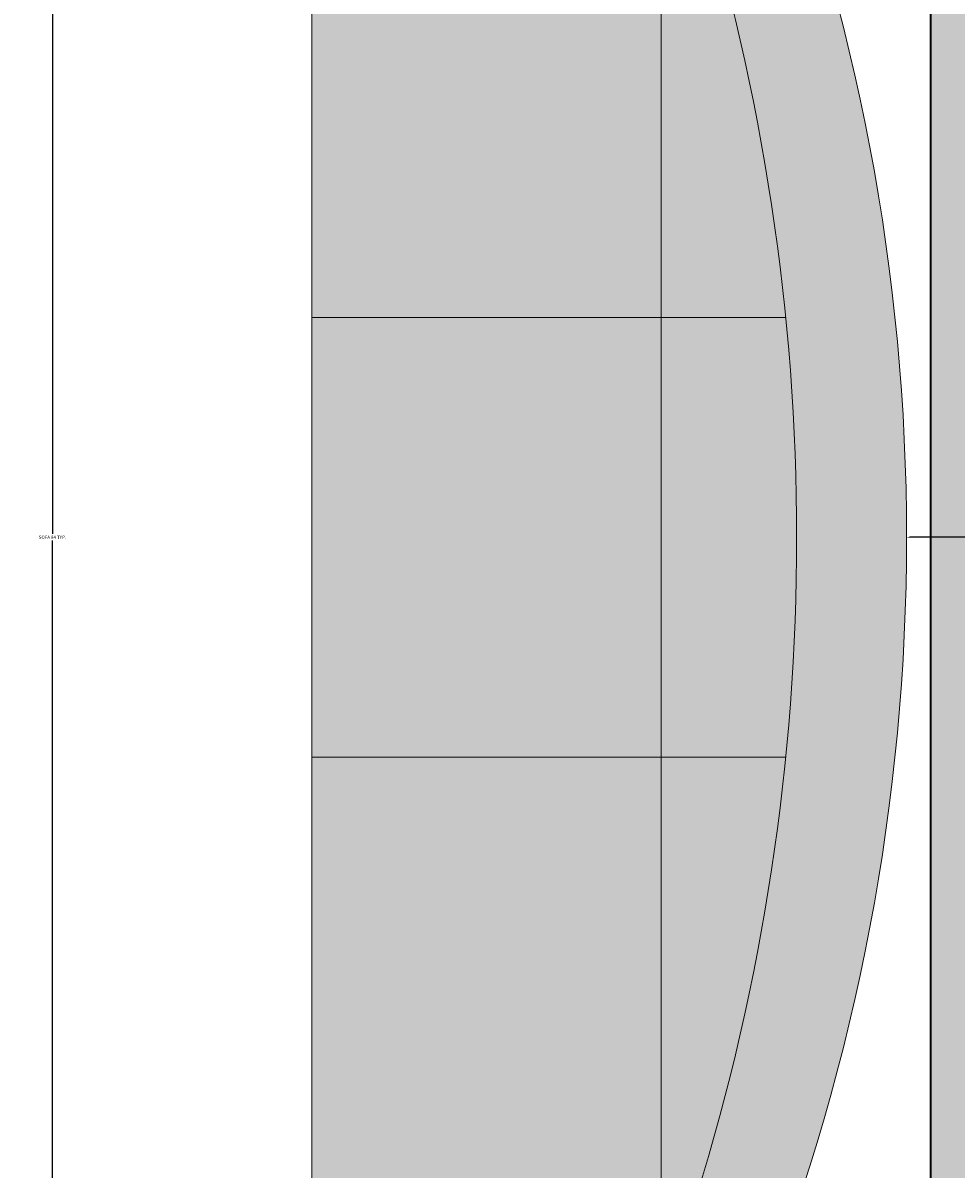
# Model space of a CAD drawing. Units: inches. Extents: x 2549 to 3108, y 1683 to 2362.
# Tile 27 of 30: x 2985 to 3036, y 2018 to 2080. Entities that reach past the tile are written whole.
import ezdxf

# ---------------------------------------------------------------- set-up
doc = ezdxf.new("R2010")
doc.units = ezdxf.units.IN
for name, color, linetype, lineweight in [('A-ANNO-DIMS', 2, 'Continuous', 18), ('A-FURN', 8, 'Continuous', 18), ('A-FURN-PATT', 9, 'Continuous', 13), ('A-WALL', 7, 'Continuous', 35), ('A-WALL-PATT', 89, 'Continuous', 13)]:
    doc.layers.add(name, color=color, linetype=linetype, lineweight=lineweight)
doc.layers.add('C-PKNG-VEHI-PATT', color=251, linetype='Continuous', lineweight=13, true_color=0x636466)
doc.layers.add('C-PVMT-PATT', color=9, linetype='Continuous', lineweight=13, true_color=0xc7c8ca)
doc.styles.get("Standard").update_dxf_attribs({"font": 'arial.ttf'})
doc.dimstyles.get("Standard").update_dxf_attribs({"dimtxt": 0.18, "dimasz": 0.18, "dimexe": 0.18, "dimexo": 0.0625, "dimgap": 0.09, "dimtad": 0, "dimtih": 1, "dimtoh": 1, "dimdec": 4, "dimzin": 0, "dimdsep": 46, "dimtxsty": 'Standard', "dimcen": 0.09, "dimadec": 0, "dimazin": 0, "dimtfac": 1, "dimtdec": 4, "dimtofl": 0, "dimtmove": 0, "dimatfit": 3, "dimfxl": 1, "dimtolj": 1, "dimtzin": 0, "dimarcsym": 0})

# ---------------------------------------------------------------- blocks, each defined once
blk = doc.blocks.new('Sofa - Roundback 7 ft.')
for p, q in [((-12.00002, -32.4421), (-12.00003, -6.5971)), ((11.99997, -32.4421), (11.99998, -6.5971)), ((-35.999844, -13.3819), (35.9998, -13.3819)), ((-36.000027, -32.4421), (35.99998, -32.4421))]:
    blk.add_line(p, q)
for centre, radius, start, end in [((0, -114.25), 114.25, 68.43141, 111.5686), ((-0.00001, -127.1968), 121.1968, 72.72033, 107.2797)]:
    blk.add_arc(centre, radius, start, end)
blk = doc.blocks.new('*D16')
at = {"layer": 'A-ANNO-DIMS', "color": 0, "lineweight": -2, "transparency": 16777216}
for p, q in [((2999.284, 2094.091), (2986.567, 2094.091)), ((2986.747, 2093.911), (2986.747, 2052.274)), ((2986.747, 2010.271), (2986.747, 2051.907)), ((2999.284, 2010.091), (2986.567, 2010.091))]:
    blk.add_line(p, q, dxfattribs=at)
at = {"layer": 'A-ANNO-DIMS', "color": 0, "transparency": 16777216}
for points in [[(2986.717, 2093.911), (2986.777, 2093.911), (2986.747, 2094.091)], [(2986.717, 2010.271), (2986.777, 2010.271), (2986.747, 2010.091)]]:
    blk.add_solid(points, dxfattribs=at)
at = {"layer": 'Defpoints', "color": 0, "transparency": 16777216}
for p in [(2999.347, 2094.091), (2986.747, 2010.091), (2999.347, 2010.091)]:
    blk.add_point(p, dxfattribs=at)
at = {"layer": 'A-ANNO-DIMS', "color": 0, "transparency": 16777216, "insert": (2986.747, 2052.091), "char_height": 0.18, "attachment_point": 5}
blk.add_mtext('\\A1;SOFA 84 TYP.', dxfattribs=at)
blk = doc.blocks.new('*D46')
at = {"layer": 'A-ANNO-DIMS', "color": 0, "lineweight": -2, "transparency": 16777216}
for p, q in [((2812.643, 2140.461), (2812.643, 1683.444)), ((3034.643, 2134.461), (3034.643, 1683.444)), ((2812.823, 1683.624), (2923.353, 1683.624)), ((3034.463, 1683.624), (2923.932, 1683.624))]:
    blk.add_line(p, q, dxfattribs=at)
at = {"layer": 'A-ANNO-DIMS', "color": 0, "transparency": 16777216}
for points in [[(2812.823, 1683.654), (2812.823, 1683.594), (2812.643, 1683.624)], [(3034.463, 1683.654), (3034.463, 1683.594), (3034.643, 1683.624)]]:
    blk.add_solid(points, dxfattribs=at)
at = {"layer": 'Defpoints', "color": 0, "transparency": 16777216}
for p in [(2812.643, 2140.524), (3034.643, 2134.524), (3034.643, 1683.624)]:
    blk.add_point(p, dxfattribs=at)
at = {"layer": 'A-ANNO-DIMS', "color": 0, "transparency": 16777216, "insert": (2923.643, 1683.624), "char_height": 0.18, "attachment_point": 5}
blk.add_mtext('\\A1;222', dxfattribs=at)
blk = doc.blocks.new('*D57')
at = {"layer": 'A-ANNO-DIMS', "color": 0, "lineweight": -2, "transparency": 16777216}
for p, q in [((2965.935, 1936.586), (2965.935, 2362.323)), ((2966.115, 2362.143), (2999.912, 2362.143)), ((3034.463, 2362.143), (3000.666, 2362.143)), ((3034.643, 1936.586), (3034.643, 2362.323))]:
    blk.add_line(p, q, dxfattribs=at)
at = {"layer": 'A-ANNO-DIMS', "color": 0, "transparency": 16777216}
for points in [[(2966.115, 2362.173), (2966.115, 2362.113), (2965.935, 2362.143)], [(3034.463, 2362.173), (3034.463, 2362.113), (3034.643, 2362.143)]]:
    blk.add_solid(points, dxfattribs=at)
at = {"layer": 'Defpoints', "color": 0, "transparency": 16777216}
for p in [(3034.643, 2362.143), (2965.935, 1936.524), (3034.643, 1936.524)]:
    blk.add_point(p, dxfattribs=at)
at = {"layer": 'A-ANNO-DIMS', "color": 0, "transparency": 16777216, "insert": (3000.289, 2362.143), "char_height": 0.18, "attachment_point": 5}
blk.add_mtext('\\A1;68.71', dxfattribs=at)
blk = doc.blocks.new('*D64')
at = {"layer": 'A-ANNO-DIMS', "color": 0, "lineweight": -2, "transparency": 16777216}
for p, q in [((2919.007, 2052.091), (2919.187, 2052.091)), ((2919.097, 2052.001), (2919.097, 2052.181)), ((3101.897, 2052.091), (3033.527, 2052.091))]:
    blk.add_line(p, q, dxfattribs=at)
at = {"layer": 'A-ANNO-DIMS', "color": 0, "transparency": 16777216}
blk.add_solid([(3033.527, 2052.121), (3033.527, 2052.061), (3033.347, 2052.091)], dxfattribs=at)
at = {"layer": 'Defpoints', "color": 0, "transparency": 16777216}
for p in [(2919.097, 2052.091), (3033.347, 2052.091)]:
    blk.add_point(p, dxfattribs=at)
at = {"layer": 'A-ANNO-DIMS', "color": 0, "transparency": 16777216, "insert": (3102.642, 2052.091), "char_height": 0.18, "attachment_point": 5}
blk.add_mtext('\\A1;2X R114.25', dxfattribs=at)

msp = doc.modelspace()

# ---------------------------------------------------------------- hatches: boundary and pattern name
at = {"layer": 'A-FURN-PATT', "transparency": 33554684}
h = msp.add_hatch(color=256, dxfattribs=at)
h.dxf.hatch_style = 1
h.paths.add_polyline_path([(2927.5085, 2119.0252, -0.1519478), (2999.5085, 2119.0252), (2999.5085, 2096.4953), (3005.5085, 2096.4953), (3005.5085, 2122.4953, 0.1904762), (2921.5085, 2122.4953), (2921.5085, 2096.4953), (2927.5085, 2096.4953)])
h.paths.add_polyline_path([(2951.5085, 2117.1134), (2927.5085, 2117.1134), (2927.5085, 2098.0532), (2951.5085, 2098.0532)], flags=17)
h.paths.add_polyline_path([(2975.5085, 2117.1134), (2951.5085, 2117.1134), (2951.5085, 2098.0532), (2975.5085, 2098.0532)], flags=17)
h.paths.add_polyline_path([(2975.5085, 2123.8998, 0.0496282), (2951.5085, 2123.8998), (2951.5085, 2117.1134), (2975.5085, 2117.1134)], flags=17)
h.paths.add_polyline_path([(2951.5085, 2123.8998, 0.0506466), (2927.5085, 2119.0252), (2927.5085, 2117.1134), (2951.5085, 2117.1134)], flags=17)
h.paths.add_polyline_path([(2975.5085, 2123.8998), (2975.5085, 2117.1134), (2999.5085, 2117.1134), (2999.5085, 2119.0252, 0.0506467)], flags=17)
h.paths.add_polyline_path([(2999.5085, 2117.1134), (2975.5085, 2117.1134), (2975.5085, 2098.0532), (2999.5085, 2098.0532)], flags=17)
h.paths.add_polyline_path([(3019.9651, 2088.0905), (3000.9049, 2088.0905), (3000.9049, 2064.0905), (3019.9651, 2064.0905)], flags=17)
h.paths.add_polyline_path([(3025.347, 2094.0905), (2999.347, 2094.0905), (2999.347, 2088.0905), (3021.8769, 2088.0905, -0.1519478), (3021.8769, 2016.0905), (2999.347, 2016.0905), (2999.347, 2010.0905), (3025.347, 2010.0905, 0.1904762)])
h.paths.add_polyline_path([(3021.8769, 2088.0905), (3019.9651, 2088.0905), (3019.9651, 2064.0905), (3026.7514, 2064.0905, 0.0506466)], flags=17)
h.paths.add_polyline_path([(3026.7514, 2064.0905), (3019.9651, 2064.0905), (3019.9651, 2040.0905), (3026.7514, 2040.0905, 0.0496282)], flags=17)
h.paths.add_polyline_path([(3019.9651, 2064.0905), (3000.9049, 2064.0905), (3000.9049, 2040.0905), (3019.9651, 2040.0905)], flags=17)
h.paths.add_polyline_path([(3019.9651, 2040.0905), (3000.9049, 2040.0905), (3000.9049, 2016.0905), (3019.9651, 2016.0905)], flags=17)
h.paths.add_polyline_path([(3026.7514, 2040.0905), (3019.9651, 2040.0905), (3019.9651, 2016.0905), (3021.8769, 2016.0905, 0.0506467)], flags=17)
at = {"layer": 'A-WALL-PATT'}
h = msp.add_hatch(color=256, dxfattribs=at)
h.dxf.hatch_style = 1
h.paths.add_polyline_path([(2638.6427, 2272.5237), (3034.6427, 2272.5237), (3034.6427, 1936.5237), (3043.6427, 1936.5237), (3043.6427, 2281.5237), (2629.6427, 2281.5237), (2629.6427, 2074.5237), (2812.6427, 2074.5237), (2812.6427, 2140.5237), (2785.7177, 2140.5237), (2785.7177, 2134.5237), (2806.6427, 2134.5237), (2806.6427, 2080.5237), (2638.6427, 2080.5237)])
h.paths.add_polyline_path([(2638.6427, 1972.5237), (2662.6427, 1972.5237), (2662.6427, 2041.0557), (2653.6427, 2041.0557), (2653.6427, 1978.5237), (2629.6427, 1978.5237), (2629.6427, 1795.5237), (2662.6427, 1795.5237), (2881.6427, 1795.5237), (2881.6427, 1936.5237), (2965.9351, 1936.5237), (2965.9351, 1974.5439), (2959.9351, 1974.5439), (2959.9351, 1945.5237), (2881.6427, 1945.5237), (2872.6427, 1945.5237), (2872.6427, 1804.5237), (2662.6427, 1804.5237), (2638.6427, 1804.5237)])
at = {"layer": 'C-PKNG-VEHI-PATT'}
h = msp.add_hatch(color=256, dxfattribs=at)
h.dxf.hatch_style = 1
edge = h.paths.add_edge_path()
edge.add_ellipse((2935.7258, 1791.964), major_axis=(-50.66, 0), ratio=0.8423039, start_angle=248.165046, end_angle=265.722579)
edge.add_line((2938.911, 1834.5507), (2925.8653, 1834.5507))
edge.add_ellipse((2929.0505, 1791.964), major_axis=(50.66, 0), ratio=0.8423039, start_angle=94.277421, end_angle=111.834954)
edge.add_line((2912.8508, 1832.3947), (2914.2044, 1822.2495))
edge.add_ellipse((2930.6538, 1783.1023), major_axis=(-49.3014, 0), ratio=0.8423039, start_angle=-85.12993, end_angle=-67.208085, ccw=False)
edge.add_line((2927.1247, 1824.5225), (2937.6516, 1824.5225))
edge.add_ellipse((2934.1225, 1783.1023), major_axis=(49.3014, 0), ratio=0.8423039, start_angle=67.208085, end_angle=85.12993, ccw=False)
edge.add_line((2950.5719, 1822.2495), (2951.9255, 1832.3947))
edge = h.paths.add_edge_path()
edge.add_ellipse((2903.4793, 1857.3351), major_axis=(-34.7979, 0), ratio=0.8423039, start_angle=180, end_angle=209.43857)
edge.add_ellipse((2961.297, 1857.3351), major_axis=(34.7979, 0), ratio=0.8423039, start_angle=150.56143, end_angle=180)
edge.add_line((2926.4991, 1857.3351), (2926.4991, 1843.7609))
edge.add_ellipse((2924.1251, 1844.3143), major_axis=(-0.2209, 3.9278), ratio=0.6038336, start_angle=89.002014, end_angle=253.657408, ccw=False)
edge.add_line((2921.7512, 1844.2222), (2921.7512, 1853.3975))
edge.add_line((2921.7512, 1853.3975), (2925.269, 1855.8484))
edge.add_ellipse((2925.4782, 1855.4931), major_axis=(0.4584, 0), ratio=0.8423039, start_angle=90, end_angle=134.480211, ccw=False)
edge.add_line((2925.4782, 1855.8792), (2926.4991, 1855.8792))
edge.add_line((2926.4991, 1855.8792), (2926.4991, 1857.3351))
edge.add_ellipse((2961.297, 1857.3351), major_axis=(34.7979, 0), ratio=0.8423039, start_angle=150.56143, end_angle=180, ccw=False)
edge.add_line((2932.3882, 1873.6501), (2932.3882, 1875.7801))
edge.add_ellipse((2932.3882, 1875.3939), major_axis=(0.4584, 0), ratio=0.8423039, start_angle=90, end_angle=127.93313)
edge.add_line((2932.1366, 1875.7167), (2928.5915, 1873.7564))
edge.add_ellipse((2899.9271, 2002.4692), major_axis=(155.4756, 0), ratio=0.84230387, start_angle=-80.743434, end_angle=-77.445067, ccw=False)
edge.add_ellipse((2949.4402, 1715.2151), major_axis=(-189.1422, 0), ratio=0.84230387, start_angle=-79.790461, end_angle=-77.555373)
edge.add_ellipse((3300.3614, 1852.5642), major_axis=(-386.1662, 0), ratio=0.84230387, start_angle=-2.863715, end_angle=2.198541)
edge.add_ellipse((2929.0505, 1792.5159), major_axis=(-55.6192, 0), ratio=0.8423039, start_angle=-85.917589, end_angle=-72.280047, ccw=False)
edge.add_line((2925.7129, 1839.2798), (2939.0634, 1839.2798))
edge.add_ellipse((2935.7258, 1792.5159), major_axis=(55.6192, 0), ratio=0.8423039, start_angle=72.280047, end_angle=85.917589, ccw=False)
edge.add_ellipse((2564.4149, 1852.5642), major_axis=(-386.1662, 0), ratio=0.84230387, start_angle=177.801459, end_angle=182.863715)
edge.add_ellipse((2915.3361, 1715.2151), major_axis=(189.1422, 0), ratio=0.84230387, start_angle=77.555373, end_angle=79.790461)
edge.add_ellipse((2964.8492, 2002.4692), major_axis=(-155.4756, 0), ratio=0.84230387, start_angle=77.445067, end_angle=80.743434, ccw=False)
edge.add_line((2936.1848, 1873.7564), (2932.6397, 1875.7167))
edge.add_ellipse((2932.3882, 1875.3939), major_axis=(0.4584, 0), ratio=0.8423039, start_angle=52.06687, end_angle=90)
edge.add_line((2932.3882, 1875.7801), (2932.3882, 1873.6501))
edge.add_ellipse((2903.4793, 1857.3351), major_axis=(-34.7979, 0), ratio=0.8423039, start_angle=180, end_angle=209.43857, ccw=False)
edge.add_line((2938.2772, 1857.3351), (2938.2772, 1855.8792))
edge.add_line((2938.2772, 1855.8792), (2939.4059, 1855.8792))
edge.add_ellipse((2939.2981, 1855.4931), major_axis=(-0.4584, 0), ratio=0.8423039, start_angle=225.519789, end_angle=270, ccw=False)
edge.add_line((2939.5903, 1855.7906), (2943.0251, 1853.3975))
edge.add_line((2943.0251, 1853.3975), (2943.0251, 1844.2222))
edge.add_ellipse((2940.6512, 1844.3143), major_axis=(0.2209, 3.9278), ratio=0.6038336, start_angle=106.342592, end_angle=270.997986, ccw=False)
edge.add_line((2938.2772, 1843.7609), (2938.2772, 1857.3351))
edge = h.paths.add_edge_path()
edge.add_ellipse((2932.3882, 1865.1973), major_axis=(91.081, 0), ratio=0.8423039, start_angle=256.401865, end_angle=283.598135, ccw=False)
edge.add_line((2914.2044, 1790.0239), (2914.2044, 1778.3622))
edge.add_ellipse((2932.3882, 1853.5356), major_axis=(91.081, 0), ratio=0.8423039, start_angle=256.401865, end_angle=283.598135)
edge.add_line((2950.5719, 1778.3622), (2950.5719, 1790.0239))
edge = h.paths.add_edge_path()
edge.add_ellipse((2948.7383, 1772.3145), major_axis=(1.8336, 0), ratio=0.8423039, start_angle=0, end_angle=90)
edge.add_line((2948.7383, 1773.859), (2916.038, 1773.859))
edge.add_ellipse((2916.038, 1772.3145), major_axis=(1.8336, 0), ratio=0.8423039, start_angle=90, end_angle=180)
edge.add_line((2914.2044, 1772.3145), (2914.2044, 1760.2558))
edge.add_line((2914.2044, 1760.2558), (2950.5719, 1760.2558))
edge.add_line((2950.5719, 1760.2558), (2950.5719, 1772.3145))
h.paths.add_polyline_path([(2748.8496, 2101.6383), (2798.148, 2101.6383), (2798.148, 2111.4248), (2748.8496, 2111.4248)], flags=9)
h.paths.add_polyline_path([(2685.2081, 2101.489), (2719.3253, 2101.489), (2719.3253, 2111.2819), (2685.2081, 2111.2819)], flags=9)
h.paths.add_polyline_path([(2814.6852, 1907.1328), (2847.8384, 1907.1328), (2847.8384, 1916.9258), (2814.6852, 1916.9258)], flags=9)
h.paths.add_polyline_path([(2814.3906, 1835.5864), (2848.0172, 1835.5864), (2848.0172, 1845.3794), (2814.3906, 1845.3794)], flags=9)
h.paths.add_polyline_path([(2800.5245, 1759.1674), (2853.7435, 1759.1674), (2853.7435, 1768.954), (2800.5245, 1768.954)], flags=9)
h.paths.add_polyline_path([(2972.4611, 1807.3305), (3015.3943, 1807.3305), (3015.3943, 1817.117), (2972.4611, 1817.117)], flags=9)
h.paths.add_polyline_path([(2902.3327, 1888.6731), (2937.9131, 1888.6731), (2937.9131, 1898.4661), (2902.3327, 1898.4661)], flags=9)
h.paths.add_polyline_path([(2712.1779, 1878.9039), (2754.1257, 1878.9039), (2754.1257, 1888.6904), (2712.1779, 1888.6904)], flags=9)
h.paths.add_polyline_path([(2614.0056, 2012.812), (2650.0251, 2012.812), (2650.0251, 2022.4371), (2614.0056, 2022.4371)], flags=9)
h.paths.add_polyline_path([(2713.3129, 2003.1645), (2747.4237, 2003.1645), (2747.4237, 2012.951), (2713.3129, 2012.951)], flags=9)
h.paths.add_polyline_path([(2950.1379, 2001.6934), (2982.2992, 2001.6934), (2982.2992, 2011.48), (2950.1379, 2011.48)], flags=9)
h.paths.add_polyline_path([(2940.864, 2238.5537), (2997.5066, 2238.5537), (2997.5066, 2248.3466), (2940.864, 2248.3466)], flags=9)
h.paths.add_polyline_path([(2821.5457, 2202.8348), (2855.663, 2202.8348), (2855.663, 2212.6278), (2821.5457, 2212.6278)], flags=9)
h.paths.add_polyline_path([(2661.8026, 2238.6249), (2718.4451, 2238.6249), (2718.4451, 2248.4179), (2661.8026, 2248.4179)], flags=9)
at = {"layer": 'C-PVMT-PATT'}
h = msp.add_hatch(color=256, dxfattribs=at)
h.dxf.hatch_style = 1
h.paths.add_polyline_path([(3067.6427, 2305.5237), (2605.6427, 2305.5237), (2605.6427, 2074.5237), (2629.6427, 2074.5237), (2629.6427, 2281.5237), (3043.6427, 2281.5237), (3043.6427, 1885.5237), (3043.6427, 1872.8745), (3031.1672, 1872.8745), (3031.1672, 1862.5731), (2995.8054, 1862.5731), (2995.8054, 1872.8745), (2983.1752, 1872.8745), (2983.1752, 1885.5237), (2881.6427, 1885.5237), (2881.6427, 1795.5237), (2751.0977, 1795.5237), (2751.0977, 1761.5237), (2786.1577, 1761.5237), (2786.1577, 1723.5237), (2881.84, 1723.5237), (2881.84, 1714.5237), (3067.6427, 1714.5237), (3067.6427, 1723.5237)])
edge = h.paths.add_edge_path(flags=16)
edge.add_ellipse((2949.4402, 1710.9683), major_axis=(-194.1014, 0), ratio=0.84230387, start_angle=-77.874034, end_angle=-76.219471, ccw=False)
edge.add_ellipse((2949.4402, 1715.2151), major_axis=(-189.1422, 0), ratio=0.84230387, start_angle=-79.790461, end_angle=-77.555373, ccw=False)
edge.add_ellipse((2899.9271, 2002.4692), major_axis=(155.4756, 0), ratio=0.84230387, start_angle=-80.743434, end_angle=-77.445067)
edge.add_line((2928.5915, 1873.7564), (2932.3882, 1875.8558))
edge.add_line((2932.3882, 1875.8558), (2936.1848, 1873.7564))
edge.add_ellipse((2964.8492, 2002.4692), major_axis=(-155.4756, 0), ratio=0.84230387, start_angle=77.445067, end_angle=80.743434)
edge.add_ellipse((2915.3361, 1715.2151), major_axis=(189.1422, 0), ratio=0.84230387, start_angle=77.555373, end_angle=79.790461, ccw=False)
edge.add_ellipse((2915.3361, 1710.9683), major_axis=(-194.1014, 0), ratio=0.84230387, start_angle=256.219471, end_angle=257.874034, ccw=False)
edge.add_ellipse((2628.2871, 1850.2612), major_axis=(-327.2532, 0), ratio=0.84230387, start_angle=182.17995, end_angle=183.650428, ccw=False)
edge.add_ellipse((2955.5637, 1861.9334), major_axis=(-0.9168, 0), ratio=0.8423039, start_angle=180, end_angle=270, ccw=False)
edge.add_line((2956.4805, 1862.3857), (2956.4805, 1846.4866))
edge.add_ellipse((2955.5637, 1846.939), major_axis=(-0.9168, 0), ratio=0.8423039, start_angle=90, end_angle=180, ccw=False)
edge.add_ellipse((-3607.0606, 1835.832), major_axis=(-6562.6242, 0), ratio=0.84230387, start_angle=179.61613322, end_angle=180.09022909, ccw=False)
edge.add_ellipse((2955.5637, 1791.0926), major_axis=(0.9168, 0), ratio=0.8423039, start_angle=0, end_angle=90, ccw=False)
edge.add_line((2956.4805, 1791.545), (2956.4805, 1775.6459))
edge.add_ellipse((2955.5637, 1776.0982), major_axis=(0.9168, 0), ratio=0.8423039, start_angle=270, end_angle=360, ccw=False)
edge.add_ellipse((-3607.0606, 1835.832), major_axis=(-6562.6242, 0), ratio=0.84230387, start_angle=179.3813568, end_angle=179.47172853, ccw=False)
edge.add_ellipse((2954.5907, 1763.8768), major_axis=(-1.3752, 0), ratio=0.8423039, start_angle=179.371763, end_angle=248.464757, ccw=False)
edge.add_ellipse((-3607.519, 1835.832), major_axis=(-6564.0409, 0), ratio=0.842303863, start_angle=179.35344594, end_angle=179.37176282, ccw=False)
edge.add_ellipse((2952.6829, 1761.8002), major_axis=(3.2503, 0), ratio=0.8423039, start_angle=-90, end_angle=-0.646554, ccw=False)
edge.add_line((2952.6829, 1759.0625), (2912.0934, 1759.0625))
edge.add_ellipse((2912.0934, 1761.8002), major_axis=(3.2503, 0), ratio=0.8423039, start_angle=180.646554, end_angle=270, ccw=False)
edge.add_ellipse((9472.2953, 1835.832), major_axis=(-6564.0409, 0), ratio=0.842303871, start_angle=0.62823722, end_angle=0.6465541, ccw=False)
edge.add_ellipse((2910.1856, 1763.8768), major_axis=(1.3752, 0), ratio=0.8423039, start_angle=111.535244, end_angle=180.628237, ccw=False)
edge.add_ellipse((9471.8369, 1835.832), major_axis=(-6562.6242, 0), ratio=0.84230387, start_angle=0.52827147, end_angle=0.6465541, ccw=False)
edge.add_ellipse((2909.2126, 1776.0982), major_axis=(-0.9168, 0), ratio=0.8423039, start_angle=0, end_angle=90, ccw=False)
edge.add_line((2908.2958, 1775.6459), (2908.2958, 1791.545))
edge.add_ellipse((2909.2126, 1791.0926), major_axis=(-0.9168, 0), ratio=0.8423039, start_angle=-90, end_angle=0, ccw=False)
edge.add_ellipse((9471.8369, 1835.832), major_axis=(-6562.6242, 0), ratio=0.84230387, start_angle=-0.09022909, end_angle=0.38386678, ccw=False)
edge.add_ellipse((2909.2126, 1846.939), major_axis=(-0.9168, 0), ratio=0.8423039, start_angle=0, end_angle=90, ccw=False)
edge.add_line((2908.2958, 1846.4866), (2908.2958, 1862.3857))
edge.add_ellipse((2909.2126, 1861.9334), major_axis=(0.9168, 0), ratio=0.8423039, start_angle=90, end_angle=180, ccw=False)
edge.add_ellipse((3236.4892, 1850.2612), major_axis=(327.2532, 0), ratio=0.84230387, start_angle=176.349572, end_angle=177.82005, ccw=False)
edge = h.paths.add_edge_path(flags=0)
edge.add_ellipse((2903.4793, 1857.3351), major_axis=(-34.7979, 0), ratio=0.8423039, start_angle=180, end_angle=209.43857, ccw=False)
edge.add_line((2938.2772, 1857.3351), (2938.2772, 1855.8792))
edge.add_line((2938.2772, 1855.8792), (2939.4631, 1855.8792))
edge.add_line((2939.4631, 1855.8792), (2943.0251, 1853.3975))
edge.add_line((2943.0251, 1853.3975), (2943.0251, 1844.2222))
edge.add_ellipse((2940.6512, 1844.3143), major_axis=(0.2209, 3.9278), ratio=0.6038336, start_angle=106.342592, end_angle=270.997986, ccw=False)
edge.add_line((2938.2772, 1843.7609), (2938.2772, 1857.3351))
edge.add_ellipse((2903.4793, 1857.3351), major_axis=(-34.7979, 0), ratio=0.8423039, start_angle=180, end_angle=209.43857)
edge.add_ellipse((2961.297, 1857.3351), major_axis=(34.7979, 0), ratio=0.8423039, start_angle=150.56143, end_angle=180)
edge.add_line((2926.4991, 1857.3351), (2926.4991, 1843.7609))
edge.add_ellipse((2924.1251, 1844.3143), major_axis=(-0.2209, 3.9278), ratio=0.6038336, start_angle=89.002014, end_angle=253.657408, ccw=False)
edge.add_line((2921.7512, 1844.2222), (2921.7512, 1853.3975))
edge.add_line((2921.7512, 1853.3975), (2925.3132, 1855.8792))
edge.add_line((2925.3132, 1855.8792), (2926.4991, 1855.8792))
edge.add_line((2926.4991, 1855.8792), (2926.4991, 1857.3351))
edge.add_ellipse((2961.297, 1857.3351), major_axis=(34.7979, 0), ratio=0.8423039, start_angle=150.56143, end_angle=180, ccw=False)
edge = h.paths.add_edge_path(flags=0)
edge.add_ellipse((2929.0505, 1791.964), major_axis=(50.66, 0), ratio=0.8423039, start_angle=94.277421, end_angle=111.834954, ccw=False)
edge.add_line((2925.8653, 1834.5507), (2938.911, 1834.5507))
edge.add_ellipse((2935.7258, 1791.964), major_axis=(-50.66, 0), ratio=0.8423039, start_angle=248.165046, end_angle=265.722579, ccw=False)
edge.add_line((2951.9255, 1832.3947), (2950.5719, 1822.2495))
edge.add_ellipse((2934.1225, 1783.1023), major_axis=(49.3014, 0), ratio=0.8423039, start_angle=67.208085, end_angle=85.12993)
edge.add_line((2937.6516, 1824.5225), (2927.1247, 1824.5225))
edge.add_ellipse((2930.6538, 1783.1023), major_axis=(-49.3014, 0), ratio=0.8423039, start_angle=-85.12993, end_angle=-67.208085)
edge.add_line((2914.2044, 1822.2495), (2912.8508, 1832.3947))
edge = h.paths.add_edge_path(flags=0)
edge.add_line((2910.1338, 1829.4651), (2912.6432, 1821.2711))
edge.add_ellipse((5203.7787, 1816.4367), major_axis=(-2291.1426, 0), ratio=0.84230387, start_angle=-0.1208974, end_angle=0.3640763)
edge.add_line((2912.7012, 1801.8782), (2910.3305, 1792.5698))
edge.add_ellipse((9471.8369, 1835.832), major_axis=(-6561.7074, 0), ratio=0.84230387, start_angle=0.05559431, end_angle=0.37776419, ccw=False)
edge = h.paths.add_edge_path(flags=0)
edge.add_ellipse((-3607.0606, 1835.832), major_axis=(6561.7074, 0), ratio=0.84230387, start_angle=-0.37776419, end_angle=-0.05559431, ccw=False)
edge.add_line((2954.4458, 1792.5698), (2952.0751, 1801.8782))
edge.add_ellipse((660.9976, 1816.4367), major_axis=(2291.1426, 0), ratio=0.84230387, start_angle=-0.3640763, end_angle=0.1208974)
edge.add_line((2952.1331, 1821.2711), (2954.6425, 1829.4651))
edge = h.paths.add_edge_path(flags=0)
edge.add_ellipse((2932.3882, 1865.1973), major_axis=(91.081, 0), ratio=0.8423039, start_angle=256.401865, end_angle=283.598135)
edge.add_line((2950.5719, 1790.0239), (2950.5719, 1778.3622))
edge.add_ellipse((2932.3882, 1853.5356), major_axis=(91.081, 0), ratio=0.8423039, start_angle=256.401865, end_angle=283.598135, ccw=False)
edge.add_line((2914.2044, 1778.3622), (2914.2044, 1790.0239))
edge = h.paths.add_edge_path(flags=0)
edge.add_line((2916.038, 1773.859), (2948.7383, 1773.859))
edge.add_ellipse((2948.7383, 1772.3145), major_axis=(1.8336, 0), ratio=0.8423039, start_angle=0, end_angle=90, ccw=False)
edge.add_line((2950.5719, 1772.3145), (2950.5719, 1760.2558))
edge.add_line((2950.5719, 1760.2558), (2914.2044, 1760.2558))
edge.add_line((2914.2044, 1760.2558), (2914.2044, 1772.3145))
edge.add_ellipse((2916.038, 1772.3145), major_axis=(1.8336, 0), ratio=0.8423039, start_angle=90, end_angle=180, ccw=False)
h.paths.add_polyline_path([(2629.6427, 1978.5237), (2605.6427, 1978.5237), (2605.6427, 1723.5237), (2629.6427, 1723.5237), (2629.6427, 1795.5237)], flags=17)
h.paths.add_polyline_path([(2800.5245, 1759.1674), (2853.7435, 1759.1674), (2853.7435, 1768.954), (2800.5245, 1768.954)], flags=24)
h.paths.add_polyline_path([(2972.4611, 1807.3305), (3015.3943, 1807.3305), (3015.3943, 1817.117), (2972.4611, 1817.117)], flags=24)

# ---------------------------------------------------------------- linework, layer by layer
at = {"layer": 'A-WALL'}
msp.add_line((3034.6427, 2272.5237), (3034.6427, 1936.5237), dxfattribs=at)

# ---------------------------------------------------------------- block references
at = {"layer": 'A-FURN', "rotation": 270}
msp.add_blockref('Sofa - Roundback 7 ft.', (3033.347, 2052.0905), dxfattribs=at)

# ---------------------------------------------------------------- dimensions: what is measured, and where the dimension line sits
at = {"layer": 'A-ANNO-DIMS'}
for base, p1, p2, override, picture, middle in [((3034.6427, 2362.1425), (2965.9351, 1936.5237), (3034.6427, 1936.5237), {"dimdec": 2, "dimlfac": 1, "dimrnd": 0, "dimzin": 0, "dimdsep": 46, "dimlunit": 2}, '*D57', (3000.2889, 2362.1425)), ((3034.6427, 1683.6237), (2812.6427, 2140.5237), (3034.6427, 2134.5237), {"dimdec": 0, "dimlfac": 1, "dimrnd": 0, "dimzin": 0, "dimdsep": 46, "dimlunit": 2}, '*D46', (2923.6427, 1683.6237))]:
    dim = msp.add_linear_dim(base=base, p1=p1, p2=p2, dimstyle='Standard', override=override, dxfattribs=at)
    dim.commit()
    dim.dimension.update_dxf_attribs({"geometry": picture, "text_midpoint": middle})
dim = msp.add_linear_dim(base=(2986.747, 2010.0905), p1=(2999.347, 2094.0905), p2=(2999.347, 2010.0905), angle=270, text='SOFA <> TYP.', dimstyle='Standard', override={"dimdec": 0, "dimlfac": 1, "dimrnd": 0, "dimzin": 0, "dimdsep": 46, "dimlunit": 2}, dxfattribs=at)
dim.commit()
dim.dimension.update_dxf_attribs({"geometry": '*D16', "text_midpoint": (2986.747, 2052.0905)})
dim = msp.add_radius_dim(center=(2919.097, 2052.0905), mpoint=(3033.347, 2052.091), text='2X <>', dimstyle='Standard', override={"dimdec": 2, "dimlfac": 1, "dimrnd": 0, "dimzin": 0, "dimdsep": 46, "dimlunit": 2}, dxfattribs=at)
dim.commit()
dim.dimension.update_dxf_attribs({"geometry": '*D64', "text_midpoint": (3101.897, 2052.0913), "dimtype": 164})

doc.saveas('drawing.dxf')
